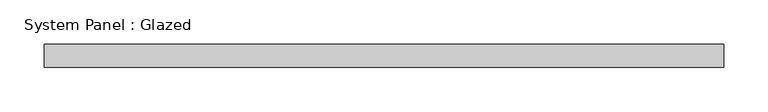
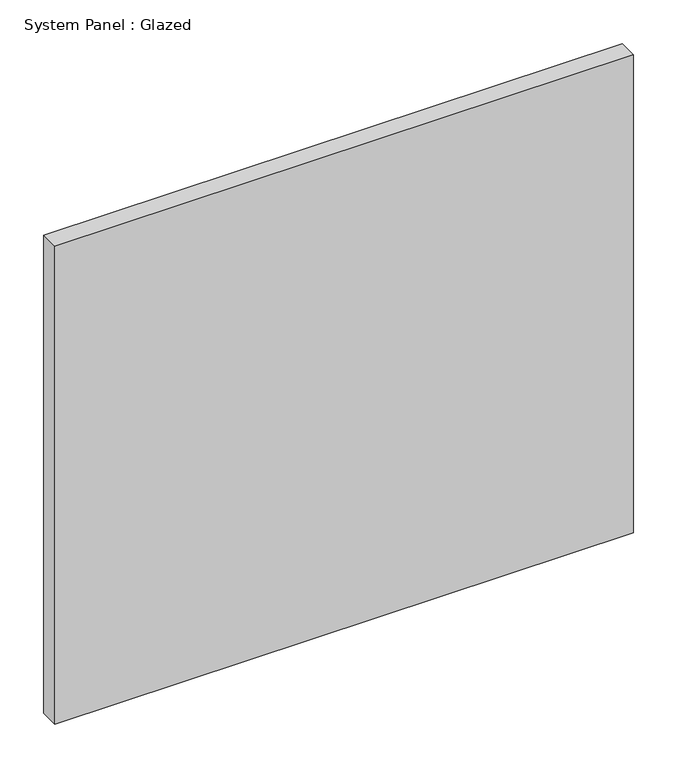
"""IFC4 building model written with IfcOpenShell, lengths in millimetres: plate geometry, System Panel : Glazed."""

from ifc_helpers import new_model, si_unit, origin, origin_with_axes, place, context, project, spatial, polyline, outline, extrude, source, transform, mapped, element, save


def system_panel_glazed_c3295151(model_context):
    return source(origin(), model_context, "Body", "SweptSolid", [
        extrude(outline(polyline([(382.0583333, 19.05), (-382.0583333, 19.05), (-382.0583333, 44.45), (382.0583333, 44.45), (382.0583333, 19.05)])), origin_with_axes(), (0.0, 0.0, 1.0), 666.75),
    ])


if __name__ == "__main__":
    model = new_model("IFC4")
    model_context = context("Model", 3, world=origin())
    ifc_project = project(units=[si_unit("LENGTHUNIT", "METRE", prefix="MILLI")], contexts=[model_context])
    site = spatial("IfcSite", under=ifc_project)
    building = spatial("IfcBuilding", under=site)
    placement = place(None, origin())
    system_panel_glazed_shape = system_panel_glazed_c3295151(model_context)
    element("IfcPlate", 1, ObjectType="System Panel : Glazed", at=placement, inside=building, context=model_context, shape_type="MappedRepresentation", body=[
        mapped(system_panel_glazed_shape, transform((0.0, 0.0, 0.0), x_axis=(1.0, 0.0, 0.0), y_axis=(0.0, 1.0, 0.0), z_axis=(0.0, 0.0, 1.0))),
    ])
    save(model, "model.ifc")

# Revit data of these elements
# Type "System Panel : Glazed"
#   Construction Type Id = "GSP4R"
#   Analytic Construction = "1/8 in Pilkington single glazing"
#   Visual Light Transmittance = 0.9
#   Solar Heat Gain Coefficient = 0.86
#   Heat Transfer Coefficient (U) = 1.18115 BTU/(h·ft²·°F)
# Element 1 (IfcPlate, "System Panel : Glazed")
#   Materials on its faces: "Glass"
# Materials
#   "Glass": class "Glass", colour RGB 0 128 192, transparency 0.75, Description = "Soda Lime Glass", Cost = 0
